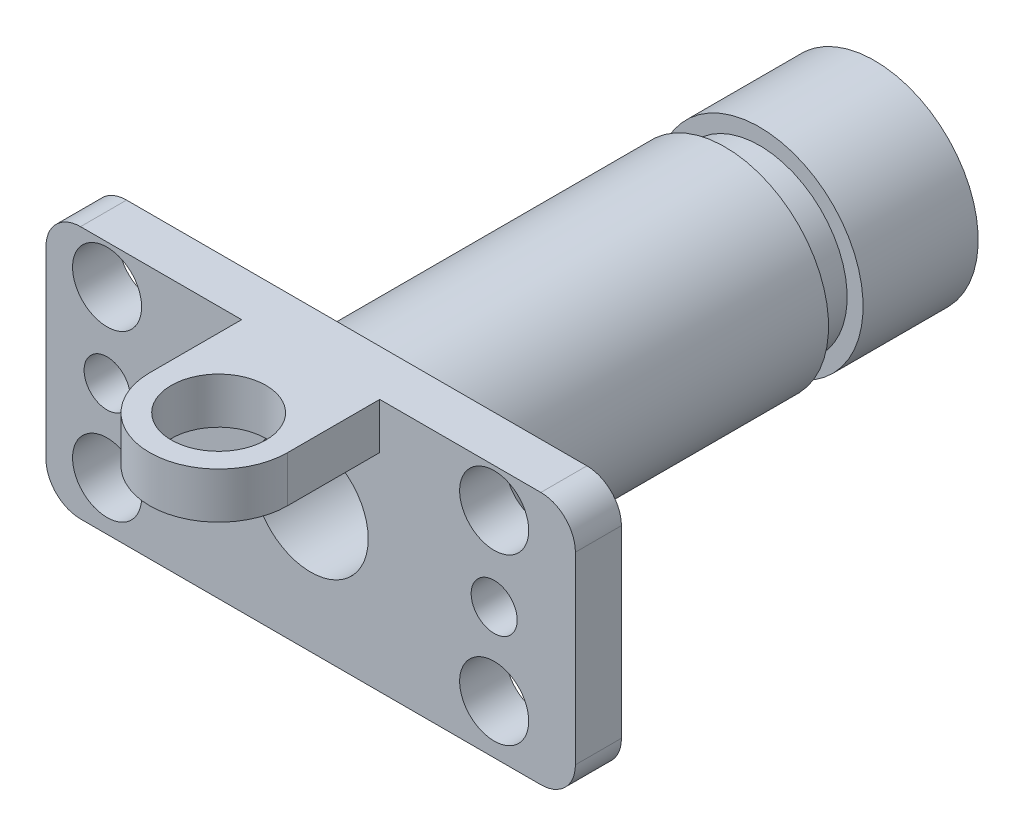
ISO-10303-21;
HEADER;
FILE_DESCRIPTION(('STEP AP214'),'2;1');
FILE_NAME('part.step','',(''),(''),'','','');
FILE_SCHEMA(('AUTOMOTIVE_DESIGN { 1 0 10303 214 1 1 1 1 }'));
ENDSEC;
DATA;
#1=APPLICATION_CONTEXT('core data for automotive mechanical design processes');
#2=APPLICATION_PROTOCOL_DEFINITION('international standard','automotive_design',2000,#1);
#3=PRODUCT_CONTEXT('',#1,'mechanical');
#4=PRODUCT('Part','Part','',(#3));
#5=PRODUCT_RELATED_PRODUCT_CATEGORY('part','',(#4));
#6=PRODUCT_DEFINITION_FORMATION('','',#4);
#7=PRODUCT_DEFINITION_CONTEXT('part definition',#1,'design');
#8=PRODUCT_DEFINITION('design','',#6,#7);
#9=PRODUCT_DEFINITION_SHAPE('','',#8);
#10=(LENGTH_UNIT() NAMED_UNIT(*) SI_UNIT(.MILLI.,.METRE.));
#11=(NAMED_UNIT(*) PLANE_ANGLE_UNIT() SI_UNIT($,.RADIAN.));
#12=(NAMED_UNIT(*) SI_UNIT($,.STERADIAN.) SOLID_ANGLE_UNIT());
#13=UNCERTAINTY_MEASURE_WITH_UNIT(LENGTH_MEASURE(1.E-05),#10,'distance_accuracy_value','');
#14=(GEOMETRIC_REPRESENTATION_CONTEXT(3) GLOBAL_UNCERTAINTY_ASSIGNED_CONTEXT((#13)) GLOBAL_UNIT_ASSIGNED_CONTEXT((#10,
#11,#12)) REPRESENTATION_CONTEXT('',''));
#15=CARTESIAN_POINT('',(0.,0.,0.));
#16=DIRECTION('',(0.,0.,1.));
#17=DIRECTION('',(1.,0.,0.));
#18=AXIS2_PLACEMENT_3D('',#15,#16,#17);
#19=CARTESIAN_POINT('',(0.,0.,10.));
#20=DIRECTION('',(0.,1.,0.));
#21=DIRECTION('',(0.,0.,1.));
#22=AXIS2_PLACEMENT_3D('',#19,#20,#21);
#23=PLANE('',#22);
#24=DIRECTION('',(1.,0.,0.));
#25=VECTOR('',#24,1.);
#26=CARTESIAN_POINT('',(0.,0.,0.));
#27=LINE('',#26,#25);
#28=CARTESIAN_POINT('',(-50.,0.,0.));
#29=VERTEX_POINT('',#28);
#30=CARTESIAN_POINT('',(50.,0.,0.));
#31=VERTEX_POINT('',#30);
#32=EDGE_CURVE('E97',#29,#31,#27,.T.);
#33=ORIENTED_EDGE('',*,*,#32,.T.);
#34=DIRECTION('',(0.,0.,-1.));
#35=VECTOR('',#34,1.);
#36=CARTESIAN_POINT('',(50.,0.,10.));
#37=LINE('',#36,#35);
#38=CARTESIAN_POINT('',(50.,0.,10.));
#39=VERTEX_POINT('',#38);
#40=EDGE_CURVE('E179',#39,#31,#37,.T.);
#41=ORIENTED_EDGE('',*,*,#40,.F.);
#42=DIRECTION('',(1.,0.,0.));
#43=VECTOR('',#42,1.);
#44=CARTESIAN_POINT('',(0.,0.,10.));
#45=LINE('',#44,#43);
#46=CARTESIAN_POINT('',(-50.,0.,10.));
#47=VERTEX_POINT('',#46);
#48=EDGE_CURVE('E101',#47,#39,#45,.T.);
#49=ORIENTED_EDGE('',*,*,#48,.F.);
#50=DIRECTION('',(0.,0.,-1.));
#51=VECTOR('',#50,1.);
#52=CARTESIAN_POINT('',(-50.,0.,10.));
#53=LINE('',#52,#51);
#54=EDGE_CURVE('E149',#47,#29,#53,.T.);
#55=ORIENTED_EDGE('',*,*,#54,.T.);
#56=EDGE_LOOP('',(#33,#41,#49,#55));
#57=FACE_BOUND('',#56,.T.);
#58=ADVANCED_FACE('F39',(#57),#23,.F.);
#59=CARTESIAN_POINT('',(50.,7.5,10.));
#60=DIRECTION('',(0.,0.,-1.));
#61=DIRECTION('',(-1.,0.,0.));
#62=AXIS2_PLACEMENT_3D('',#59,#60,#61);
#63=CYLINDRICAL_SURFACE('',#62,7.5);
#64=CARTESIAN_POINT('',(50.,7.5,0.));
#65=DIRECTION('',(0.,0.,1.));
#66=DIRECTION('',(1.,0.,0.));
#67=AXIS2_PLACEMENT_3D('',#64,#65,#66);
#68=CIRCLE('',#67,7.5);
#69=CARTESIAN_POINT('',(57.5,7.5,0.));
#70=VERTEX_POINT('',#69);
#71=EDGE_CURVE('E151',#31,#70,#68,.T.);
#72=ORIENTED_EDGE('',*,*,#71,.T.);
#73=DIRECTION('',(0.,0.,-1.));
#74=VECTOR('',#73,1.);
#75=CARTESIAN_POINT('',(57.5,7.5,10.));
#76=LINE('',#75,#74);
#77=CARTESIAN_POINT('',(57.5,7.5,10.));
#78=VERTEX_POINT('',#77);
#79=EDGE_CURVE('E180',#78,#70,#76,.T.);
#80=ORIENTED_EDGE('',*,*,#79,.F.);
#81=CARTESIAN_POINT('',(50.,7.5,10.));
#82=DIRECTION('',(0.,0.,1.));
#83=DIRECTION('',(1.,0.,0.));
#84=AXIS2_PLACEMENT_3D('',#81,#82,#83);
#85=CIRCLE('',#84,7.5);
#86=EDGE_CURVE('E228',#39,#78,#85,.T.);
#87=ORIENTED_EDGE('',*,*,#86,.F.);
#88=ORIENTED_EDGE('',*,*,#40,.T.);
#89=EDGE_LOOP('',(#72,#80,#87,#88));
#90=FACE_BOUND('',#89,.T.);
#91=ADVANCED_FACE('F302',(#90),#63,.T.);
#92=CARTESIAN_POINT('',(57.5,7.5,10.));
#93=DIRECTION('',(-1.,0.,0.));
#94=DIRECTION('',(0.,0.,1.));
#95=AXIS2_PLACEMENT_3D('',#92,#93,#94);
#96=PLANE('',#95);
#97=DIRECTION('',(0.,1.,0.));
#98=VECTOR('',#97,1.);
#99=CARTESIAN_POINT('',(57.5,7.5,0.));
#100=LINE('',#99,#98);
#101=CARTESIAN_POINT('',(57.5,47.5,0.));
#102=VERTEX_POINT('',#101);
#103=EDGE_CURVE('E159',#70,#102,#100,.T.);
#104=ORIENTED_EDGE('',*,*,#103,.T.);
#105=DIRECTION('',(0.,0.,-1.));
#106=VECTOR('',#105,1.);
#107=CARTESIAN_POINT('',(57.5,47.5,10.));
#108=LINE('',#107,#106);
#109=CARTESIAN_POINT('',(57.5,47.5,10.));
#110=VERTEX_POINT('',#109);
#111=EDGE_CURVE('E172',#110,#102,#108,.T.);
#112=ORIENTED_EDGE('',*,*,#111,.F.);
#113=DIRECTION('',(0.,1.,0.));
#114=VECTOR('',#113,1.);
#115=CARTESIAN_POINT('',(57.5,7.5,10.));
#116=LINE('',#115,#114);
#117=EDGE_CURVE('E226',#78,#110,#116,.T.);
#118=ORIENTED_EDGE('',*,*,#117,.F.);
#119=ORIENTED_EDGE('',*,*,#79,.T.);
#120=EDGE_LOOP('',(#104,#112,#118,#119));
#121=FACE_BOUND('',#120,.T.);
#122=ADVANCED_FACE('F307',(#121),#96,.F.);
#123=CARTESIAN_POINT('',(50.,47.5,10.));
#124=DIRECTION('',(0.,0.,-1.));
#125=DIRECTION('',(-1.,0.,0.));
#126=AXIS2_PLACEMENT_3D('',#123,#124,#125);
#127=CYLINDRICAL_SURFACE('',#126,7.5);
#128=CARTESIAN_POINT('',(50.,47.5,0.));
#129=DIRECTION('',(0.,0.,1.));
#130=DIRECTION('',(1.,0.,0.));
#131=AXIS2_PLACEMENT_3D('',#128,#129,#130);
#132=CIRCLE('',#131,7.5);
#133=CARTESIAN_POINT('',(50.,55.,0.));
#134=VERTEX_POINT('',#133);
#135=EDGE_CURVE('E160',#102,#134,#132,.T.);
#136=ORIENTED_EDGE('',*,*,#135,.T.);
#137=DIRECTION('',(0.,0.,-1.));
#138=VECTOR('',#137,1.);
#139=CARTESIAN_POINT('',(50.,55.,10.));
#140=LINE('',#139,#138);
#141=CARTESIAN_POINT('',(50.,55.,10.));
#142=VERTEX_POINT('',#141);
#143=EDGE_CURVE('E171',#142,#134,#140,.T.);
#144=ORIENTED_EDGE('',*,*,#143,.F.);
#145=CARTESIAN_POINT('',(50.,47.5,10.));
#146=DIRECTION('',(0.,0.,1.));
#147=DIRECTION('',(1.,0.,0.));
#148=AXIS2_PLACEMENT_3D('',#145,#146,#147);
#149=CIRCLE('',#148,7.5);
#150=EDGE_CURVE('E229',#110,#142,#149,.T.);
#151=ORIENTED_EDGE('',*,*,#150,.F.);
#152=ORIENTED_EDGE('',*,*,#111,.T.);
#153=EDGE_LOOP('',(#136,#144,#151,#152));
#154=FACE_BOUND('',#153,.T.);
#155=ADVANCED_FACE('F316',(#154),#127,.T.);
#156=CARTESIAN_POINT('',(-50.,55.,10.));
#157=DIRECTION('',(0.,-1.,0.));
#158=DIRECTION('',(0.,0.,-1.));
#159=AXIS2_PLACEMENT_3D('',#156,#157,#158);
#160=PLANE('',#159);
#161=CARTESIAN_POINT('',(0.,55.,30.));
#162=DIRECTION('',(0.,-1.,0.));
#163=DIRECTION('',(0.,0.,-1.));
#164=AXIS2_PLACEMENT_3D('',#161,#162,#163);
#165=CIRCLE('',#164,10.2866996569793);
#166=CARTESIAN_POINT('',(0.,55.,19.7133003430207));
#167=VERTEX_POINT('',#166);
#168=EDGE_CURVE('E527',#167,#167,#165,.T.);
#169=ORIENTED_EDGE('',*,*,#168,.T.);
#170=EDGE_LOOP('',(#169));
#171=FACE_BOUND('',#170,.T.);
#172=DIRECTION('',(-1.,0.,0.));
#173=VECTOR('',#172,1.);
#174=CARTESIAN_POINT('',(-50.,55.,0.));
#175=LINE('',#174,#173);
#176=CARTESIAN_POINT('',(-50.,55.,0.));
#177=VERTEX_POINT('',#176);
#178=EDGE_CURVE('E157',#134,#177,#175,.T.);
#179=ORIENTED_EDGE('',*,*,#178,.T.);
#180=DIRECTION('',(0.,0.,-1.));
#181=VECTOR('',#180,1.);
#182=CARTESIAN_POINT('',(-50.,55.,10.));
#183=LINE('',#182,#181);
#184=CARTESIAN_POINT('',(-50.,55.,10.));
#185=VERTEX_POINT('',#184);
#186=EDGE_CURVE('E145',#185,#177,#183,.T.);
#187=ORIENTED_EDGE('',*,*,#186,.F.);
#188=DIRECTION('',(-1.,0.,0.));
#189=VECTOR('',#188,1.);
#190=CARTESIAN_POINT('',(-50.,55.,10.));
#191=LINE('',#190,#189);
#192=CARTESIAN_POINT('',(-15.,55.,10.));
#193=VERTEX_POINT('',#192);
#194=EDGE_CURVE('E126',#193,#185,#191,.T.);
#195=ORIENTED_EDGE('',*,*,#194,.F.);
#196=DIRECTION('',(0.,0.,1.));
#197=VECTOR('',#196,1.);
#198=CARTESIAN_POINT('',(-15.,55.,10.));
#199=LINE('',#198,#197);
#200=CARTESIAN_POINT('',(-15.,55.,30.));
#201=VERTEX_POINT('',#200);
#202=EDGE_CURVE('E54',#193,#201,#199,.T.);
#203=ORIENTED_EDGE('',*,*,#202,.T.);
#204=CARTESIAN_POINT('',(0.,55.,30.));
#205=DIRECTION('',(0.,1.,0.));
#206=DIRECTION('',(0.,0.,1.));
#207=AXIS2_PLACEMENT_3D('',#204,#205,#206);
#208=CIRCLE('',#207,15.);
#209=CARTESIAN_POINT('',(15.,55.,30.));
#210=VERTEX_POINT('',#209);
#211=EDGE_CURVE('E247',#201,#210,#208,.T.);
#212=ORIENTED_EDGE('',*,*,#211,.T.);
#213=DIRECTION('',(0.,0.,-1.));
#214=VECTOR('',#213,1.);
#215=CARTESIAN_POINT('',(15.,55.,10.));
#216=LINE('',#215,#214);
#217=CARTESIAN_POINT('',(15.,55.,10.));
#218=VERTEX_POINT('',#217);
#219=EDGE_CURVE('E246',#210,#218,#216,.T.);
#220=ORIENTED_EDGE('',*,*,#219,.T.);
#221=EDGE_CURVE('E131',#142,#218,#191,.T.);
#222=ORIENTED_EDGE('',*,*,#221,.F.);
#223=ORIENTED_EDGE('',*,*,#143,.T.);
#224=EDGE_LOOP('',(#179,#187,#195,#203,#212,#220,#222,#223));
#225=FACE_BOUND('',#224,.T.);
#226=ADVANCED_FACE('F245',(#171,#225),#160,.F.);
#227=CARTESIAN_POINT('',(-50.,47.5,10.));
#228=DIRECTION('',(0.,0.,-1.));
#229=DIRECTION('',(-1.,0.,0.));
#230=AXIS2_PLACEMENT_3D('',#227,#228,#229);
#231=CYLINDRICAL_SURFACE('',#230,7.5);
#232=CARTESIAN_POINT('',(-50.,47.5,0.));
#233=DIRECTION('',(0.,0.,1.));
#234=DIRECTION('',(1.,0.,0.));
#235=AXIS2_PLACEMENT_3D('',#232,#233,#234);
#236=CIRCLE('',#235,7.5);
#237=CARTESIAN_POINT('',(-57.5,47.5,0.));
#238=VERTEX_POINT('',#237);
#239=EDGE_CURVE('E138',#177,#238,#236,.T.);
#240=ORIENTED_EDGE('',*,*,#239,.T.);
#241=DIRECTION('',(0.,0.,-1.));
#242=VECTOR('',#241,1.);
#243=CARTESIAN_POINT('',(-57.5,47.5,10.));
#244=LINE('',#243,#242);
#245=CARTESIAN_POINT('',(-57.5,47.5,10.));
#246=VERTEX_POINT('',#245);
#247=EDGE_CURVE('E139',#246,#238,#244,.T.);
#248=ORIENTED_EDGE('',*,*,#247,.F.);
#249=CARTESIAN_POINT('',(-50.,47.5,10.));
#250=DIRECTION('',(0.,0.,1.));
#251=DIRECTION('',(1.,0.,0.));
#252=AXIS2_PLACEMENT_3D('',#249,#250,#251);
#253=CIRCLE('',#252,7.5);
#254=EDGE_CURVE('E119',#185,#246,#253,.T.);
#255=ORIENTED_EDGE('',*,*,#254,.F.);
#256=ORIENTED_EDGE('',*,*,#186,.T.);
#257=EDGE_LOOP('',(#240,#248,#255,#256));
#258=FACE_BOUND('',#257,.T.);
#259=ADVANCED_FACE('F136',(#258),#231,.T.);
#260=CARTESIAN_POINT('',(-57.5,7.5,10.));
#261=DIRECTION('',(1.,0.,0.));
#262=DIRECTION('',(0.,0.,-1.));
#263=AXIS2_PLACEMENT_3D('',#260,#261,#262);
#264=PLANE('',#263);
#265=DIRECTION('',(0.,-1.,0.));
#266=VECTOR('',#265,1.);
#267=CARTESIAN_POINT('',(-57.5,7.5,0.));
#268=LINE('',#267,#266);
#269=CARTESIAN_POINT('',(-57.5,7.5,0.));
#270=VERTEX_POINT('',#269);
#271=EDGE_CURVE('E161',#238,#270,#268,.T.);
#272=ORIENTED_EDGE('',*,*,#271,.T.);
#273=DIRECTION('',(0.,0.,-1.));
#274=VECTOR('',#273,1.);
#275=CARTESIAN_POINT('',(-57.5,7.5,10.));
#276=LINE('',#275,#274);
#277=CARTESIAN_POINT('',(-57.5,7.5,10.));
#278=VERTEX_POINT('',#277);
#279=EDGE_CURVE('E141',#278,#270,#276,.T.);
#280=ORIENTED_EDGE('',*,*,#279,.F.);
#281=DIRECTION('',(0.,-1.,0.));
#282=VECTOR('',#281,1.);
#283=CARTESIAN_POINT('',(-57.5,7.5,10.));
#284=LINE('',#283,#282);
#285=EDGE_CURVE('E127',#246,#278,#284,.T.);
#286=ORIENTED_EDGE('',*,*,#285,.F.);
#287=ORIENTED_EDGE('',*,*,#247,.T.);
#288=EDGE_LOOP('',(#272,#280,#286,#287));
#289=FACE_BOUND('',#288,.T.);
#290=ADVANCED_FACE('F143',(#289),#264,.F.);
#291=CARTESIAN_POINT('',(-50.,7.5,10.));
#292=DIRECTION('',(0.,0.,-1.));
#293=DIRECTION('',(-1.,0.,0.));
#294=AXIS2_PLACEMENT_3D('',#291,#292,#293);
#295=CYLINDRICAL_SURFACE('',#294,7.5);
#296=CARTESIAN_POINT('',(-50.,7.5,0.));
#297=DIRECTION('',(0.,0.,1.));
#298=DIRECTION('',(1.,0.,0.));
#299=AXIS2_PLACEMENT_3D('',#296,#297,#298);
#300=CIRCLE('',#299,7.5);
#301=EDGE_CURVE('E164',#270,#29,#300,.T.);
#302=ORIENTED_EDGE('',*,*,#301,.T.);
#303=ORIENTED_EDGE('',*,*,#54,.F.);
#304=CARTESIAN_POINT('',(-50.,7.5,10.));
#305=DIRECTION('',(0.,0.,1.));
#306=DIRECTION('',(1.,0.,0.));
#307=AXIS2_PLACEMENT_3D('',#304,#305,#306);
#308=CIRCLE('',#307,7.5);
#309=EDGE_CURVE('E61',#278,#47,#308,.T.);
#310=ORIENTED_EDGE('',*,*,#309,.F.);
#311=ORIENTED_EDGE('',*,*,#279,.T.);
#312=EDGE_LOOP('',(#302,#303,#310,#311));
#313=FACE_BOUND('',#312,.T.);
#314=ADVANCED_FACE('F287',(#313),#295,.T.);
#315=CARTESIAN_POINT('',(-50.,7.5,10.));
#316=DIRECTION('',(0.,0.,1.));
#317=DIRECTION('',(1.,0.,0.));
#318=AXIS2_PLACEMENT_3D('',#315,#316,#317);
#319=PLANE('',#318);
#320=DIRECTION('',(0.,1.,0.));
#321=VECTOR('',#320,1.);
#322=CARTESIAN_POINT('',(15.,45.,10.));
#323=LINE('',#322,#321);
#324=CARTESIAN_POINT('',(15.,45.,10.));
#325=VERTEX_POINT('',#324);
#326=EDGE_CURVE('E232',#325,#218,#323,.T.);
#327=ORIENTED_EDGE('',*,*,#326,.F.);
#328=DIRECTION('',(-1.,0.,0.));
#329=VECTOR('',#328,1.);
#330=CARTESIAN_POINT('',(0.,45.,10.));
#331=LINE('',#330,#329);
#332=CARTESIAN_POINT('',(-15.,45.,10.));
#333=VERTEX_POINT('',#332);
#334=EDGE_CURVE('E252',#325,#333,#331,.T.);
#335=ORIENTED_EDGE('',*,*,#334,.T.);
#336=DIRECTION('',(0.,1.,0.));
#337=VECTOR('',#336,1.);
#338=CARTESIAN_POINT('',(-15.,45.,10.));
#339=LINE('',#338,#337);
#340=EDGE_CURVE('E262',#333,#193,#339,.T.);
#341=ORIENTED_EDGE('',*,*,#340,.T.);
#342=ORIENTED_EDGE('',*,*,#194,.T.);
#343=ORIENTED_EDGE('',*,*,#254,.T.);
#344=ORIENTED_EDGE('',*,*,#285,.T.);
#345=ORIENTED_EDGE('',*,*,#309,.T.);
#346=ORIENTED_EDGE('',*,*,#48,.T.);
#347=ORIENTED_EDGE('',*,*,#86,.T.);
#348=ORIENTED_EDGE('',*,*,#117,.T.);
#349=ORIENTED_EDGE('',*,*,#150,.T.);
#350=ORIENTED_EDGE('',*,*,#221,.T.);
#351=EDGE_LOOP('',(#327,#335,#341,#342,#343,#344,#345,#346,#347,#348,#349,#350));
#352=FACE_BOUND('',#351,.T.);
#353=CARTESIAN_POINT('',(-44.2306146906631,46.5294505064485,10.));
#354=DIRECTION('',(0.,0.,1.));
#355=DIRECTION('',(1.,0.,0.));
#356=AXIS2_PLACEMENT_3D('',#353,#354,#355);
#357=CIRCLE('',#356,7.5);
#358=CARTESIAN_POINT('',(-36.7306146906631,46.5294505064485,10.));
#359=VERTEX_POINT('',#358);
#360=EDGE_CURVE('E256',#359,#359,#357,.T.);
#361=ORIENTED_EDGE('',*,*,#360,.F.);
#362=EDGE_LOOP('',(#361));
#363=FACE_BOUND('',#362,.T.);
#364=CARTESIAN_POINT('',(-44.2306146906631,28.4000415780081,10.));
#365=DIRECTION('',(0.,0.,1.));
#366=DIRECTION('',(1.,0.,0.));
#367=AXIS2_PLACEMENT_3D('',#364,#365,#366);
#368=CIRCLE('',#367,5.);
#369=CARTESIAN_POINT('',(-39.2306146906631,28.4000415780081,10.));
#370=VERTEX_POINT('',#369);
#371=EDGE_CURVE('E280',#370,#370,#368,.T.);
#372=ORIENTED_EDGE('',*,*,#371,.F.);
#373=EDGE_LOOP('',(#372));
#374=FACE_BOUND('',#373,.T.);
#375=CARTESIAN_POINT('',(-44.2306146906631,10.6563647544281,10.));
#376=DIRECTION('',(0.,0.,1.));
#377=DIRECTION('',(1.,0.,0.));
#378=AXIS2_PLACEMENT_3D('',#375,#376,#377);
#379=CIRCLE('',#378,7.5);
#380=CARTESIAN_POINT('',(-36.7306146906631,10.6563647544281,10.));
#381=VERTEX_POINT('',#380);
#382=EDGE_CURVE('E274',#381,#381,#379,.T.);
#383=ORIENTED_EDGE('',*,*,#382,.F.);
#384=EDGE_LOOP('',(#383));
#385=FACE_BOUND('',#384,.T.);
#386=CARTESIAN_POINT('',(39.8589841689115,10.6563647544281,10.));
#387=DIRECTION('',(0.,0.,1.));
#388=DIRECTION('',(1.,0.,0.));
#389=AXIS2_PLACEMENT_3D('',#386,#387,#388);
#390=CIRCLE('',#389,7.5);
#391=CARTESIAN_POINT('',(47.3589841689115,10.6563647544281,10.));
#392=VERTEX_POINT('',#391);
#393=EDGE_CURVE('E272',#392,#392,#390,.T.);
#394=ORIENTED_EDGE('',*,*,#393,.F.);
#395=EDGE_LOOP('',(#394));
#396=FACE_BOUND('',#395,.T.);
#397=CARTESIAN_POINT('',(39.8589841689115,28.4000415780081,10.));
#398=DIRECTION('',(0.,0.,1.));
#399=DIRECTION('',(1.,0.,0.));
#400=AXIS2_PLACEMENT_3D('',#397,#398,#399);
#401=CIRCLE('',#400,5.);
#402=CARTESIAN_POINT('',(44.8589841689115,28.4000415780081,10.));
#403=VERTEX_POINT('',#402);
#404=EDGE_CURVE('E270',#403,#403,#401,.T.);
#405=ORIENTED_EDGE('',*,*,#404,.F.);
#406=EDGE_LOOP('',(#405));
#407=FACE_BOUND('',#406,.T.);
#408=CARTESIAN_POINT('',(39.8589841689115,46.5294505064485,10.));
#409=DIRECTION('',(0.,0.,1.));
#410=DIRECTION('',(1.,0.,0.));
#411=AXIS2_PLACEMENT_3D('',#408,#409,#410);
#412=CIRCLE('',#411,7.5);
#413=CARTESIAN_POINT('',(47.3589841689115,46.5294505064485,10.));
#414=VERTEX_POINT('',#413);
#415=EDGE_CURVE('E190',#414,#414,#412,.T.);
#416=ORIENTED_EDGE('',*,*,#415,.F.);
#417=EDGE_LOOP('',(#416));
#418=FACE_BOUND('',#417,.T.);
#419=CARTESIAN_POINT('',(0.,27.5,10.));
#420=DIRECTION('',(0.,0.,1.));
#421=DIRECTION('',(1.,0.,0.));
#422=AXIS2_PLACEMENT_3D('',#419,#420,#421);
#423=CIRCLE('',#422,12.5);
#424=CARTESIAN_POINT('',(12.5,27.5,10.));
#425=VERTEX_POINT('',#424);
#426=EDGE_CURVE('E197',#425,#425,#423,.T.);
#427=ORIENTED_EDGE('',*,*,#426,.F.);
#428=EDGE_LOOP('',(#427));
#429=FACE_BOUND('',#428,.T.);
#430=ADVANCED_FACE('F124',(#352,#363,#374,#385,#396,#407,#418,#429),#319,.T.);
#431=CARTESIAN_POINT('',(-50.,7.5,0.));
#432=DIRECTION('',(0.,0.,1.));
#433=DIRECTION('',(1.,0.,0.));
#434=AXIS2_PLACEMENT_3D('',#431,#432,#433);
#435=PLANE('',#434);
#436=CARTESIAN_POINT('',(-44.2306146906631,46.5294505064485,0.));
#437=DIRECTION('',(0.,0.,1.));
#438=DIRECTION('',(1.,0.,0.));
#439=AXIS2_PLACEMENT_3D('',#436,#437,#438);
#440=CIRCLE('',#439,7.5);
#441=CARTESIAN_POINT('',(-36.7306146906631,46.5294505064485,0.));
#442=VERTEX_POINT('',#441);
#443=EDGE_CURVE('E45',#442,#442,#440,.T.);
#444=ORIENTED_EDGE('',*,*,#443,.T.);
#445=EDGE_LOOP('',(#444));
#446=FACE_BOUND('',#445,.T.);
#447=CARTESIAN_POINT('',(-44.2306146906631,28.4000415780081,0.));
#448=DIRECTION('',(0.,0.,1.));
#449=DIRECTION('',(1.,0.,0.));
#450=AXIS2_PLACEMENT_3D('',#447,#448,#449);
#451=CIRCLE('',#450,5.);
#452=CARTESIAN_POINT('',(-39.2306146906631,28.4000415780081,0.));
#453=VERTEX_POINT('',#452);
#454=EDGE_CURVE('E193',#453,#453,#451,.T.);
#455=ORIENTED_EDGE('',*,*,#454,.T.);
#456=EDGE_LOOP('',(#455));
#457=FACE_BOUND('',#456,.T.);
#458=CARTESIAN_POINT('',(-44.2306146906631,10.6563647544281,0.));
#459=DIRECTION('',(0.,0.,1.));
#460=DIRECTION('',(1.,0.,0.));
#461=AXIS2_PLACEMENT_3D('',#458,#459,#460);
#462=CIRCLE('',#461,7.5);
#463=CARTESIAN_POINT('',(-36.7306146906631,10.6563647544281,0.));
#464=VERTEX_POINT('',#463);
#465=EDGE_CURVE('E194',#464,#464,#462,.T.);
#466=ORIENTED_EDGE('',*,*,#465,.T.);
#467=EDGE_LOOP('',(#466));
#468=FACE_BOUND('',#467,.T.);
#469=CARTESIAN_POINT('',(39.8589841689115,10.6563647544281,0.));
#470=DIRECTION('',(0.,0.,1.));
#471=DIRECTION('',(1.,0.,0.));
#472=AXIS2_PLACEMENT_3D('',#469,#470,#471);
#473=CIRCLE('',#472,7.5);
#474=CARTESIAN_POINT('',(47.3589841689115,10.6563647544281,0.));
#475=VERTEX_POINT('',#474);
#476=EDGE_CURVE('E188',#475,#475,#473,.T.);
#477=ORIENTED_EDGE('',*,*,#476,.T.);
#478=EDGE_LOOP('',(#477));
#479=FACE_BOUND('',#478,.T.);
#480=CARTESIAN_POINT('',(39.8589841689115,28.4000415780081,0.));
#481=DIRECTION('',(0.,0.,1.));
#482=DIRECTION('',(1.,0.,0.));
#483=AXIS2_PLACEMENT_3D('',#480,#481,#482);
#484=CIRCLE('',#483,5.);
#485=CARTESIAN_POINT('',(44.8589841689115,28.4000415780081,0.));
#486=VERTEX_POINT('',#485);
#487=EDGE_CURVE('E187',#486,#486,#484,.T.);
#488=ORIENTED_EDGE('',*,*,#487,.T.);
#489=EDGE_LOOP('',(#488));
#490=FACE_BOUND('',#489,.T.);
#491=CARTESIAN_POINT('',(39.8589841689115,46.5294505064485,0.));
#492=DIRECTION('',(0.,0.,1.));
#493=DIRECTION('',(1.,0.,0.));
#494=AXIS2_PLACEMENT_3D('',#491,#492,#493);
#495=CIRCLE('',#494,7.5);
#496=CARTESIAN_POINT('',(47.3589841689115,46.5294505064485,0.));
#497=VERTEX_POINT('',#496);
#498=EDGE_CURVE('E182',#497,#497,#495,.T.);
#499=ORIENTED_EDGE('',*,*,#498,.T.);
#500=EDGE_LOOP('',(#499));
#501=FACE_BOUND('',#500,.T.);
#502=CARTESIAN_POINT('',(0.,27.5,0.));
#503=DIRECTION('',(0.,0.,-1.));
#504=DIRECTION('',(-1.,0.,0.));
#505=AXIS2_PLACEMENT_3D('',#502,#503,#504);
#506=CIRCLE('',#505,22.5);
#507=CARTESIAN_POINT('',(-22.5,27.5,0.));
#508=VERTEX_POINT('',#507);
#509=EDGE_CURVE('E50',#508,#508,#506,.T.);
#510=ORIENTED_EDGE('',*,*,#509,.F.);
#511=EDGE_LOOP('',(#510));
#512=FACE_BOUND('',#511,.T.);
#513=ORIENTED_EDGE('',*,*,#32,.F.);
#514=ORIENTED_EDGE('',*,*,#301,.F.);
#515=ORIENTED_EDGE('',*,*,#271,.F.);
#516=ORIENTED_EDGE('',*,*,#239,.F.);
#517=ORIENTED_EDGE('',*,*,#178,.F.);
#518=ORIENTED_EDGE('',*,*,#135,.F.);
#519=ORIENTED_EDGE('',*,*,#103,.F.);
#520=ORIENTED_EDGE('',*,*,#71,.F.);
#521=EDGE_LOOP('',(#513,#514,#515,#516,#517,#518,#519,#520));
#522=FACE_BOUND('',#521,.T.);
#523=ADVANCED_FACE('F288',(#446,#457,#468,#479,#490,#501,#512,#522),#435,.F.);
#524=CARTESIAN_POINT('',(0.,27.5,-80.));
#525=DIRECTION('',(0.,0.,1.));
#526=DIRECTION('',(1.,0.,0.));
#527=AXIS2_PLACEMENT_3D('',#524,#525,#526);
#528=CYLINDRICAL_SURFACE('',#527,22.5);
#529=CARTESIAN_POINT('',(0.,27.5,-80.));
#530=DIRECTION('',(0.,0.,-1.));
#531=DIRECTION('',(-1.,0.,0.));
#532=AXIS2_PLACEMENT_3D('',#529,#530,#531);
#533=CIRCLE('',#532,22.5);
#534=CARTESIAN_POINT('',(-22.5,27.5,-80.));
#535=VERTEX_POINT('',#534);
#536=EDGE_CURVE('E154',#535,#535,#533,.T.);
#537=ORIENTED_EDGE('',*,*,#536,.F.);
#538=EDGE_LOOP('',(#537));
#539=FACE_BOUND('',#538,.T.);
#540=ORIENTED_EDGE('',*,*,#509,.T.);
#541=EDGE_LOOP('',(#540));
#542=FACE_BOUND('',#541,.T.);
#543=ADVANCED_FACE('F300',(#539,#542),#528,.T.);
#544=CARTESIAN_POINT('',(0.,27.5,-80.));
#545=DIRECTION('',(0.,0.,-1.));
#546=DIRECTION('',(-1.,0.,0.));
#547=AXIS2_PLACEMENT_3D('',#544,#545,#546);
#548=PLANE('',#547);
#549=CARTESIAN_POINT('',(0.,27.5,-80.));
#550=DIRECTION('',(0.,0.,-1.));
#551=DIRECTION('',(-1.,0.,0.));
#552=AXIS2_PLACEMENT_3D('',#549,#550,#551);
#553=CIRCLE('',#552,19.0385703641239);
#554=CARTESIAN_POINT('',(-19.0385703641239,27.5,-80.));
#555=VERTEX_POINT('',#554);
#556=EDGE_CURVE('E11',#555,#555,#553,.T.);
#557=ORIENTED_EDGE('',*,*,#556,.F.);
#558=EDGE_LOOP('',(#557));
#559=FACE_BOUND('',#558,.T.);
#560=ORIENTED_EDGE('',*,*,#536,.T.);
#561=EDGE_LOOP('',(#560));
#562=FACE_BOUND('',#561,.T.);
#563=ADVANCED_FACE('F349',(#559,#562),#548,.T.);
#564=CARTESIAN_POINT('',(0.,27.5,-87.5));
#565=DIRECTION('',(0.,0.,1.));
#566=DIRECTION('',(1.,0.,0.));
#567=AXIS2_PLACEMENT_3D('',#564,#565,#566);
#568=CYLINDRICAL_SURFACE('',#567,19.0385703641239);
#569=CARTESIAN_POINT('',(0.,27.5,-87.5));
#570=DIRECTION('',(0.,0.,-1.));
#571=DIRECTION('',(-1.,0.,0.));
#572=AXIS2_PLACEMENT_3D('',#569,#570,#571);
#573=CIRCLE('',#572,19.0385703641239);
#574=CARTESIAN_POINT('',(-19.0385703641239,27.5,-87.5));
#575=VERTEX_POINT('',#574);
#576=EDGE_CURVE('E218',#575,#575,#573,.T.);
#577=ORIENTED_EDGE('',*,*,#576,.F.);
#578=EDGE_LOOP('',(#577));
#579=FACE_BOUND('',#578,.T.);
#580=ORIENTED_EDGE('',*,*,#556,.T.);
#581=EDGE_LOOP('',(#580));
#582=FACE_BOUND('',#581,.T.);
#583=ADVANCED_FACE('F356',(#579,#582),#568,.T.);
#584=CARTESIAN_POINT('',(0.,27.5,-112.5));
#585=DIRECTION('',(0.,0.,1.));
#586=DIRECTION('',(1.,0.,0.));
#587=AXIS2_PLACEMENT_3D('',#584,#585,#586);
#588=CYLINDRICAL_SURFACE('',#587,22.5);
#589=CARTESIAN_POINT('',(0.,27.5,-112.5));
#590=DIRECTION('',(0.,0.,-1.));
#591=DIRECTION('',(-1.,0.,0.));
#592=AXIS2_PLACEMENT_3D('',#589,#590,#591);
#593=CIRCLE('',#592,22.5);
#594=CARTESIAN_POINT('',(-22.5,27.5,-112.5));
#595=VERTEX_POINT('',#594);
#596=EDGE_CURVE('E214',#595,#595,#593,.T.);
#597=ORIENTED_EDGE('',*,*,#596,.F.);
#598=EDGE_LOOP('',(#597));
#599=FACE_BOUND('',#598,.T.);
#600=CARTESIAN_POINT('',(0.,27.5,-87.5));
#601=DIRECTION('',(0.,0.,-1.));
#602=DIRECTION('',(-1.,0.,0.));
#603=AXIS2_PLACEMENT_3D('',#600,#601,#602);
#604=CIRCLE('',#603,22.5);
#605=CARTESIAN_POINT('',(-22.5,27.5,-87.5));
#606=VERTEX_POINT('',#605);
#607=EDGE_CURVE('E209',#606,#606,#604,.T.);
#608=ORIENTED_EDGE('',*,*,#607,.T.);
#609=EDGE_LOOP('',(#608));
#610=FACE_BOUND('',#609,.T.);
#611=ADVANCED_FACE('F370',(#599,#610),#588,.T.);
#612=CARTESIAN_POINT('',(0.,27.5,-112.5));
#613=DIRECTION('',(0.,0.,-1.));
#614=DIRECTION('',(-1.,0.,0.));
#615=AXIS2_PLACEMENT_3D('',#612,#613,#614);
#616=PLANE('',#615);
#617=ORIENTED_EDGE('',*,*,#596,.T.);
#618=EDGE_LOOP('',(#617));
#619=FACE_BOUND('',#618,.T.);
#620=ADVANCED_FACE('F376',(#619),#616,.T.);
#621=CARTESIAN_POINT('',(0.,27.5,-87.5));
#622=DIRECTION('',(0.,0.,-1.));
#623=DIRECTION('',(-1.,0.,0.));
#624=AXIS2_PLACEMENT_3D('',#621,#622,#623);
#625=PLANE('',#624);
#626=ORIENTED_EDGE('',*,*,#576,.T.);
#627=EDGE_LOOP('',(#626));
#628=FACE_BOUND('',#627,.T.);
#629=ORIENTED_EDGE('',*,*,#607,.F.);
#630=EDGE_LOOP('',(#629));
#631=FACE_BOUND('',#630,.T.);
#632=ADVANCED_FACE('F383',(#628,#631),#625,.F.);
#633=CARTESIAN_POINT('',(0.,27.5,-15.));
#634=DIRECTION('',(0.,0.,1.));
#635=DIRECTION('',(1.,0.,0.));
#636=AXIS2_PLACEMENT_3D('',#633,#634,#635);
#637=CYLINDRICAL_SURFACE('',#636,12.5);
#638=CARTESIAN_POINT('',(0.,27.5,-15.));
#639=DIRECTION('',(0.,0.,1.));
#640=DIRECTION('',(1.,0.,0.));
#641=AXIS2_PLACEMENT_3D('',#638,#639,#640);
#642=CIRCLE('',#641,12.5);
#643=CARTESIAN_POINT('',(12.5,27.5,-15.));
#644=VERTEX_POINT('',#643);
#645=EDGE_CURVE('E203',#644,#644,#642,.T.);
#646=ORIENTED_EDGE('',*,*,#645,.F.);
#647=EDGE_LOOP('',(#646));
#648=FACE_BOUND('',#647,.T.);
#649=ORIENTED_EDGE('',*,*,#426,.T.);
#650=EDGE_LOOP('',(#649));
#651=FACE_BOUND('',#650,.T.);
#652=ADVANCED_FACE('F394',(#648,#651),#637,.F.);
#653=CARTESIAN_POINT('',(0.,27.5,-15.));
#654=DIRECTION('',(0.,0.,1.));
#655=DIRECTION('',(1.,0.,0.));
#656=AXIS2_PLACEMENT_3D('',#653,#654,#655);
#657=PLANE('',#656);
#658=ORIENTED_EDGE('',*,*,#645,.T.);
#659=EDGE_LOOP('',(#658));
#660=FACE_BOUND('',#659,.T.);
#661=ADVANCED_FACE('F401',(#660),#657,.T.);
#662=CARTESIAN_POINT('',(39.8589841689115,46.5294505064485,-15.));
#663=DIRECTION('',(0.,0.,1.));
#664=DIRECTION('',(1.,0.,0.));
#665=AXIS2_PLACEMENT_3D('',#662,#663,#664);
#666=CYLINDRICAL_SURFACE('',#665,7.5);
#667=ORIENTED_EDGE('',*,*,#415,.T.);
#668=EDGE_LOOP('',(#667));
#669=FACE_BOUND('',#668,.T.);
#670=ORIENTED_EDGE('',*,*,#498,.F.);
#671=EDGE_LOOP('',(#670));
#672=FACE_BOUND('',#671,.T.);
#673=ADVANCED_FACE('F284',(#669,#672),#666,.F.);
#674=CARTESIAN_POINT('',(39.8589841689115,28.4000415780081,-15.));
#675=DIRECTION('',(0.,0.,1.));
#676=DIRECTION('',(1.,0.,0.));
#677=AXIS2_PLACEMENT_3D('',#674,#675,#676);
#678=CYLINDRICAL_SURFACE('',#677,5.);
#679=ORIENTED_EDGE('',*,*,#404,.T.);
#680=EDGE_LOOP('',(#679));
#681=FACE_BOUND('',#680,.T.);
#682=ORIENTED_EDGE('',*,*,#487,.F.);
#683=EDGE_LOOP('',(#682));
#684=FACE_BOUND('',#683,.T.);
#685=ADVANCED_FACE('F425',(#681,#684),#678,.F.);
#686=CARTESIAN_POINT('',(39.8589841689115,10.6563647544281,-15.));
#687=DIRECTION('',(0.,0.,1.));
#688=DIRECTION('',(1.,0.,0.));
#689=AXIS2_PLACEMENT_3D('',#686,#687,#688);
#690=CYLINDRICAL_SURFACE('',#689,7.5);
#691=ORIENTED_EDGE('',*,*,#393,.T.);
#692=EDGE_LOOP('',(#691));
#693=FACE_BOUND('',#692,.T.);
#694=ORIENTED_EDGE('',*,*,#476,.F.);
#695=EDGE_LOOP('',(#694));
#696=FACE_BOUND('',#695,.T.);
#697=ADVANCED_FACE('F435',(#693,#696),#690,.F.);
#698=CARTESIAN_POINT('',(-44.2306146906631,10.6563647544281,-15.));
#699=DIRECTION('',(0.,0.,1.));
#700=DIRECTION('',(1.,0.,0.));
#701=AXIS2_PLACEMENT_3D('',#698,#699,#700);
#702=CYLINDRICAL_SURFACE('',#701,7.5);
#703=ORIENTED_EDGE('',*,*,#382,.T.);
#704=EDGE_LOOP('',(#703));
#705=FACE_BOUND('',#704,.T.);
#706=ORIENTED_EDGE('',*,*,#465,.F.);
#707=EDGE_LOOP('',(#706));
#708=FACE_BOUND('',#707,.T.);
#709=ADVANCED_FACE('F441',(#705,#708),#702,.F.);
#710=CARTESIAN_POINT('',(-44.2306146906631,28.4000415780081,-15.));
#711=DIRECTION('',(0.,0.,1.));
#712=DIRECTION('',(1.,0.,0.));
#713=AXIS2_PLACEMENT_3D('',#710,#711,#712);
#714=CYLINDRICAL_SURFACE('',#713,5.);
#715=ORIENTED_EDGE('',*,*,#371,.T.);
#716=EDGE_LOOP('',(#715));
#717=FACE_BOUND('',#716,.T.);
#718=ORIENTED_EDGE('',*,*,#454,.F.);
#719=EDGE_LOOP('',(#718));
#720=FACE_BOUND('',#719,.T.);
#721=ADVANCED_FACE('F448',(#717,#720),#714,.F.);
#722=CARTESIAN_POINT('',(-44.2306146906631,46.5294505064485,-15.));
#723=DIRECTION('',(0.,0.,1.));
#724=DIRECTION('',(1.,0.,0.));
#725=AXIS2_PLACEMENT_3D('',#722,#723,#724);
#726=CYLINDRICAL_SURFACE('',#725,7.5);
#727=ORIENTED_EDGE('',*,*,#360,.T.);
#728=EDGE_LOOP('',(#727));
#729=FACE_BOUND('',#728,.T.);
#730=ORIENTED_EDGE('',*,*,#443,.F.);
#731=EDGE_LOOP('',(#730));
#732=FACE_BOUND('',#731,.T.);
#733=ADVANCED_FACE('F456',(#729,#732),#726,.F.);
#734=CARTESIAN_POINT('',(15.,45.,10.));
#735=DIRECTION('',(1.,0.,0.));
#736=DIRECTION('',(0.,0.,-1.));
#737=AXIS2_PLACEMENT_3D('',#734,#735,#736);
#738=PLANE('',#737);
#739=ORIENTED_EDGE('',*,*,#219,.F.);
#740=DIRECTION('',(0.,1.,0.));
#741=VECTOR('',#740,1.);
#742=CARTESIAN_POINT('',(15.,45.,30.));
#743=LINE('',#742,#741);
#744=CARTESIAN_POINT('',(15.,45.,30.));
#745=VERTEX_POINT('',#744);
#746=EDGE_CURVE('E258',#745,#210,#743,.T.);
#747=ORIENTED_EDGE('',*,*,#746,.F.);
#748=DIRECTION('',(0.,0.,-1.));
#749=VECTOR('',#748,1.);
#750=CARTESIAN_POINT('',(15.,45.,10.));
#751=LINE('',#750,#749);
#752=EDGE_CURVE('E266',#745,#325,#751,.T.);
#753=ORIENTED_EDGE('',*,*,#752,.T.);
#754=ORIENTED_EDGE('',*,*,#326,.T.);
#755=EDGE_LOOP('',(#739,#747,#753,#754));
#756=FACE_BOUND('',#755,.T.);
#757=ADVANCED_FACE('F467',(#756),#738,.T.);
#758=CARTESIAN_POINT('',(0.,45.,30.));
#759=DIRECTION('',(0.,1.,0.));
#760=DIRECTION('',(0.,0.,1.));
#761=AXIS2_PLACEMENT_3D('',#758,#759,#760);
#762=CYLINDRICAL_SURFACE('',#761,15.);
#763=ORIENTED_EDGE('',*,*,#211,.F.);
#764=DIRECTION('',(0.,1.,0.));
#765=VECTOR('',#764,1.);
#766=CARTESIAN_POINT('',(-15.,45.,30.));
#767=LINE('',#766,#765);
#768=CARTESIAN_POINT('',(-15.,45.,30.));
#769=VERTEX_POINT('',#768);
#770=EDGE_CURVE('E261',#769,#201,#767,.T.);
#771=ORIENTED_EDGE('',*,*,#770,.F.);
#772=CARTESIAN_POINT('',(0.,45.,30.));
#773=DIRECTION('',(0.,1.,0.));
#774=DIRECTION('',(0.,0.,1.));
#775=AXIS2_PLACEMENT_3D('',#772,#773,#774);
#776=CIRCLE('',#775,15.);
#777=EDGE_CURVE('E536',#769,#745,#776,.T.);
#778=ORIENTED_EDGE('',*,*,#777,.T.);
#779=ORIENTED_EDGE('',*,*,#746,.T.);
#780=EDGE_LOOP('',(#763,#771,#778,#779));
#781=FACE_BOUND('',#780,.T.);
#782=ADVANCED_FACE('F486',(#781),#762,.T.);
#783=CARTESIAN_POINT('',(-15.,45.,10.));
#784=DIRECTION('',(-1.,0.,0.));
#785=DIRECTION('',(0.,0.,1.));
#786=AXIS2_PLACEMENT_3D('',#783,#784,#785);
#787=PLANE('',#786);
#788=ORIENTED_EDGE('',*,*,#202,.F.);
#789=ORIENTED_EDGE('',*,*,#340,.F.);
#790=DIRECTION('',(0.,0.,1.));
#791=VECTOR('',#790,1.);
#792=CARTESIAN_POINT('',(-15.,45.,10.));
#793=LINE('',#792,#791);
#794=EDGE_CURVE('E254',#333,#769,#793,.T.);
#795=ORIENTED_EDGE('',*,*,#794,.T.);
#796=ORIENTED_EDGE('',*,*,#770,.T.);
#797=EDGE_LOOP('',(#788,#789,#795,#796));
#798=FACE_BOUND('',#797,.T.);
#799=ADVANCED_FACE('F500',(#798),#787,.T.);
#800=CARTESIAN_POINT('',(0.,45.,30.));
#801=DIRECTION('',(0.,1.,0.));
#802=DIRECTION('',(0.,0.,1.));
#803=AXIS2_PLACEMENT_3D('',#800,#801,#802);
#804=PLANE('',#803);
#805=CARTESIAN_POINT('',(0.,45.,30.));
#806=DIRECTION('',(0.,-1.,0.));
#807=DIRECTION('',(0.,0.,-1.));
#808=AXIS2_PLACEMENT_3D('',#805,#806,#807);
#809=CIRCLE('',#808,10.2866996569793);
#810=CARTESIAN_POINT('',(0.,45.,19.7133003430207));
#811=VERTEX_POINT('',#810);
#812=EDGE_CURVE('E531',#811,#811,#809,.T.);
#813=ORIENTED_EDGE('',*,*,#812,.F.);
#814=EDGE_LOOP('',(#813));
#815=FACE_BOUND('',#814,.T.);
#816=ORIENTED_EDGE('',*,*,#334,.F.);
#817=ORIENTED_EDGE('',*,*,#752,.F.);
#818=ORIENTED_EDGE('',*,*,#777,.F.);
#819=ORIENTED_EDGE('',*,*,#794,.F.);
#820=EDGE_LOOP('',(#816,#817,#818,#819));
#821=FACE_BOUND('',#820,.T.);
#822=ADVANCED_FACE('F506',(#815,#821),#804,.F.);
#823=CARTESIAN_POINT('',(0.,55.,30.));
#824=DIRECTION('',(0.,-1.,0.));
#825=DIRECTION('',(0.,0.,-1.));
#826=AXIS2_PLACEMENT_3D('',#823,#824,#825);
#827=CYLINDRICAL_SURFACE('',#826,10.2866996569793);
#828=ORIENTED_EDGE('',*,*,#168,.F.);
#829=EDGE_LOOP('',(#828));
#830=FACE_BOUND('',#829,.T.);
#831=ORIENTED_EDGE('',*,*,#812,.T.);
#832=EDGE_LOOP('',(#831));
#833=FACE_BOUND('',#832,.T.);
#834=ADVANCED_FACE('F511',(#830,#833),#827,.F.);
#835=CLOSED_SHELL('',(#58,#91,#122,#155,#226,#259,#290,#314,#430,#523,#543,#563,#583,#611,#620,
#632,#652,#661,#673,#685,#697,#709,#721,#733,#757,#782,#799,#822,#834));
#836=MANIFOLD_SOLID_BREP('B2',#835);
#837=ADVANCED_BREP_SHAPE_REPRESENTATION('',(#18,#836),#14);
#838=SHAPE_DEFINITION_REPRESENTATION(#9,#837);
ENDSEC;
END-ISO-10303-21;
